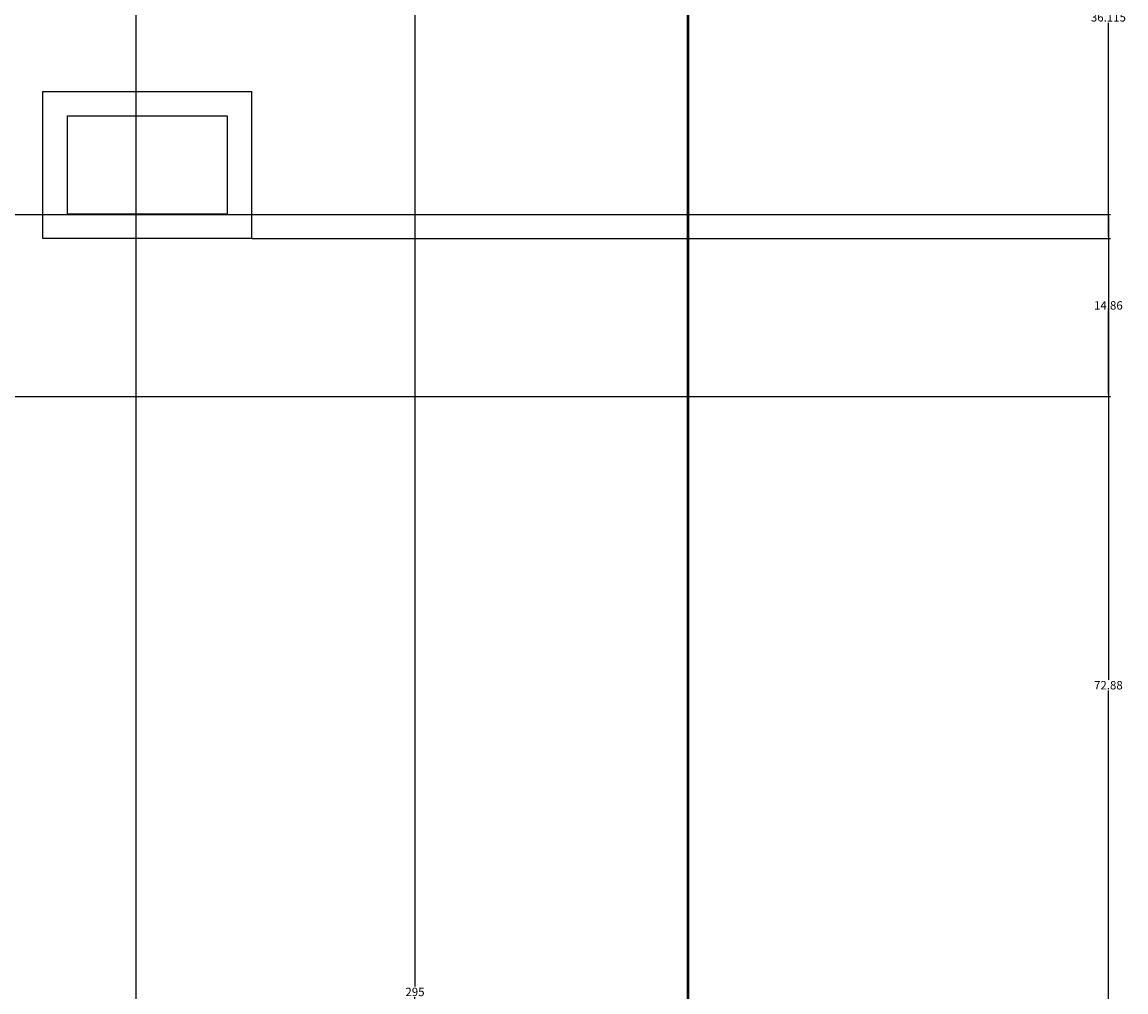
# Model space of a CAD drawing. Units: inches. Extents: x -139 to 346, y 72 to 413.
# Tile 17 of 18: x 256 to 346, y 242 to 322. Entities that reach past the tile are written whole.
import ezdxf

# ---------------------------------------------------------------- set-up
doc = ezdxf.new("R2010")
doc.units = ezdxf.units.IN
doc.header["$MEASUREMENT"] = 0
for name, color, linetype, lineweight in [('A-ANNO-DIMS', 2, 'Continuous', 18), ('A-GLAZ', 4, 'Continuous', 25), ('A-WALL', 7, 'Continuous', 50)]:
    doc.layers.add(name, color=color, linetype=linetype, lineweight=lineweight)
doc.styles.get("Standard").update_dxf_attribs({"font": 'arial.ttf'})
doc.dimstyles.get("Standard").update_dxf_attribs({"dimtxt": 0.6875, "dimasz": 0.18, "dimexe": 0.18, "dimexo": 0.0625, "dimgap": 0.09, "dimtad": 0, "dimtih": 1, "dimtoh": 1, "dimdec": 4, "dimzin": 0, "dimdsep": 46, "dimlunit": 4, "dimtxsty": 'Standard', "dimcen": 0.09, "dimadec": 0, "dimazin": 0, "dimtfac": 1, "dimtdec": 4, "dimtofl": 0, "dimtmove": 0, "dimatfit": 3, "dimfxl": 1, "dimtolj": 1, "dimtzin": 0, "dimarcsym": 0})

# ---------------------------------------------------------------- blocks, each defined once
blk = doc.blocks.new('WIN-SMALL')
for points in [[(0, 12.015), (17.035, 12.015), (17.035, 0), (0, 0)], [(2, 10.015), (15.035, 10.015), (15.035, 2), (2, 2)]]:
    blk.add_lwpolyline(points, close=True)
blk = doc.blocks.new('*D31')
at = {"layer": 'A-ANNO-DIMS', "color": 0, "lineweight": -2, "transparency": 16777216}
for p, q in [((309.827, 389.975), (287.409, 389.975)), ((287.589, 389.795), (287.589, 242.916)), ((287.589, 95.155), (287.589, 242.034)), ((309.827, 94.975), (287.409, 94.975))]:
    blk.add_line(p, q, dxfattribs=at)
at = {"layer": 'A-ANNO-DIMS', "color": 0, "transparency": 16777216}
for points in [[(287.559, 389.795), (287.619, 389.795), (287.589, 389.975)], [(287.559, 95.155), (287.619, 95.155), (287.589, 94.975)]]:
    blk.add_solid(points, dxfattribs=at)
at = {"layer": 'Defpoints', "color": 0, "transparency": 16777216}
for p in [(287.589, 389.975), (309.889, 389.975), (309.889, 94.975)]:
    blk.add_point(p, dxfattribs=at)
at = {"layer": 'A-ANNO-DIMS', "color": 0, "transparency": 16777216, "insert": (287.589, 242.475), "char_height": 0.6875, "attachment_point": 5}
blk.add_mtext('\\A1;295', dxfattribs=at)
blk = doc.blocks.new('*D34')
at = {"layer": 'A-ANNO-DIMS', "color": 0, "lineweight": -2, "transparency": 16777216}
for p, q in [((274.309, 303.94), (344.386, 303.94)), ((344.206, 303.76), (344.206, 267.941)), ((344.206, 231.241), (344.206, 267.059)), ((297.564, 231.061), (344.386, 231.061))]:
    blk.add_line(p, q, dxfattribs=at)
at = {"layer": 'A-ANNO-DIMS', "color": 0, "transparency": 16777216}
for points in [[(344.176, 303.76), (344.236, 303.76), (344.206, 303.94)], [(344.176, 231.241), (344.236, 231.241), (344.206, 231.061)]]:
    blk.add_solid(points, dxfattribs=at)
at = {"layer": 'Defpoints', "color": 0, "transparency": 16777216}
for p in [(274.247, 303.94), (344.206, 303.94), (297.501, 231.061)]:
    blk.add_point(p, dxfattribs=at)
at = {"layer": 'A-ANNO-DIMS', "color": 0, "transparency": 16777216, "insert": (344.206, 267.5), "char_height": 0.6875, "attachment_point": 5}
blk.add_mtext('\\A1;72.88', dxfattribs=at)
blk = doc.blocks.new('*D35')
at = {"layer": 'A-ANNO-DIMS', "color": 0, "lineweight": -2, "transparency": 16777216}
for p, q in [((274.309, 340.055), (344.386, 340.055)), ((344.206, 339.875), (344.206, 322.439)), ((344.206, 304.12), (344.206, 321.556)), ((274.309, 303.94), (344.386, 303.94))]:
    blk.add_line(p, q, dxfattribs=at)
at = {"layer": 'A-ANNO-DIMS', "color": 0, "transparency": 16777216}
for points in [[(344.176, 339.875), (344.236, 339.875), (344.206, 340.055)], [(344.176, 304.12), (344.236, 304.12), (344.206, 303.94)]]:
    blk.add_solid(points, dxfattribs=at)
at = {"layer": 'Defpoints', "color": 0, "transparency": 16777216}
for p in [(274.247, 340.055), (344.206, 340.055), (274.247, 303.94)]:
    blk.add_point(p, dxfattribs=at)
at = {"layer": 'A-ANNO-DIMS', "color": 0, "transparency": 16777216, "insert": (344.206, 321.998), "char_height": 0.6875, "attachment_point": 5}
blk.add_mtext('\\A1;36.115', dxfattribs=at)
blk = doc.blocks.new('*D82')
at = {"layer": 'A-ANNO-DIMS', "color": 0, "lineweight": -2, "transparency": 16777216}
for p, q in [((245.84, 184.668), (245.84, 412.455)), ((246.02, 412.275), (253.85, 412.275)), ((264.642, 412.275), (256.812, 412.275)), ((264.822, 184.668), (264.822, 412.455))]:
    blk.add_line(p, q, dxfattribs=at)
at = {"layer": 'A-ANNO-DIMS', "color": 0, "transparency": 16777216}
for points in [[(246.02, 412.305), (246.02, 412.245), (245.84, 412.275)], [(264.642, 412.305), (264.642, 412.245), (264.822, 412.275)]]:
    blk.add_solid(points, dxfattribs=at)
at = {"layer": 'Defpoints', "color": 0, "transparency": 16777216}
for p in [(264.822, 412.275), (245.84, 184.606), (264.822, 184.606)]:
    blk.add_point(p, dxfattribs=at)
at = {"layer": 'A-ANNO-DIMS', "color": 0, "transparency": 16777216, "insert": (255.331, 412.275), "char_height": 0.6875, "attachment_point": 5}
blk.add_mtext('\\A1;18.982', dxfattribs=at)
blk = doc.blocks.new('*D101')
at = {"layer": 'A-ANNO-DIMS', "color": 0, "lineweight": -2, "transparency": 16777216}
for p, q in [((110.387, 305.921), (344.386, 305.921)), ((344.206, 305.741), (344.206, 298.931)), ((344.206, 291.24), (344.206, 298.049)), ((112.713, 291.06), (344.386, 291.06))]:
    blk.add_line(p, q, dxfattribs=at)
at = {"layer": 'A-ANNO-DIMS', "color": 0, "transparency": 16777216}
for points in [[(344.176, 305.741), (344.236, 305.741), (344.206, 305.921)], [(344.176, 291.24), (344.236, 291.24), (344.206, 291.06)]]:
    blk.add_solid(points, dxfattribs=at)
at = {"layer": 'Defpoints', "color": 0, "transparency": 16777216}
for p in [(110.324, 305.921), (344.206, 305.921), (112.651, 291.06)]:
    blk.add_point(p, dxfattribs=at)
at = {"layer": 'A-ANNO-DIMS', "color": 0, "transparency": 16777216, "insert": (344.206, 298.49), "char_height": 0.6875, "attachment_point": 5}
blk.add_mtext('\\A1;14.86', dxfattribs=at)

msp = doc.modelspace()

# ---------------------------------------------------------------- linework, layer by layer
at = {"layer": 'A-WALL'}
msp.add_line((309.8894, 94.9748), (309.8894, 382.9748), dxfattribs=at)

# ---------------------------------------------------------------- block references
at = {"layer": 'A-GLAZ'}
msp.add_blockref('WIN-SMALL', (257.212, 303.9404), dxfattribs=at)

# ---------------------------------------------------------------- dimensions: what is measured, and where the dimension line sits
at = {"layer": 'A-ANNO-DIMS'}
dim = msp.add_linear_dim(base=(264.8219, 412.2748), p1=(245.8399, 184.6055), p2=(264.8219, 184.6055), dimstyle='Standard', override={"dimdec": 3, "dimlfac": 1, "dimrnd": 0, "dimzin": 0, "dimdsep": 46, "dimlunit": 2}, dxfattribs=at)
dim.commit()
dim.dimension.update_dxf_attribs({"geometry": '*D82', "text_midpoint": (255.3309, 412.2748)})
for base, p1, p2, override, picture, middle in [((287.5894, 389.9748), (309.8894, 94.9748), (309.8894, 389.9748), {"dimdec": 0, "dimlfac": 1, "dimrnd": 0, "dimzin": 0, "dimdsep": 46, "dimlunit": 2}, '*D31', (287.5894, 242.4748)), ((344.2055, 340.0548), (274.2465, 303.9402), (274.2465, 340.0548), {"dimdec": 3, "dimlfac": 1, "dimrnd": 0, "dimzin": 0, "dimdsep": 46, "dimlunit": 2}, '*D35', (344.2055, 321.9975)), ((344.2055, 305.9205), (112.6506, 291.0604), (110.3243, 305.9205), {"dimdec": 2, "dimlfac": 1, "dimrnd": 0, "dimzin": 0, "dimdsep": 46, "dimlunit": 2}, '*D101', (344.2055, 298.4905)), ((344.2055, 303.9402), (297.5013, 231.0607), (274.2465, 303.9402), {"dimdec": 2, "dimlfac": 1, "dimrnd": 0, "dimzin": 0, "dimdsep": 46, "dimlunit": 2}, '*D34', (344.2055, 267.5005))]:
    dim = msp.add_linear_dim(base=base, p1=p1, p2=p2, angle=90, dimstyle='Standard', override=override, dxfattribs=at)
    dim.commit()
    dim.dimension.update_dxf_attribs({"geometry": picture, "text_midpoint": middle})

doc.saveas('drawing.dxf')
